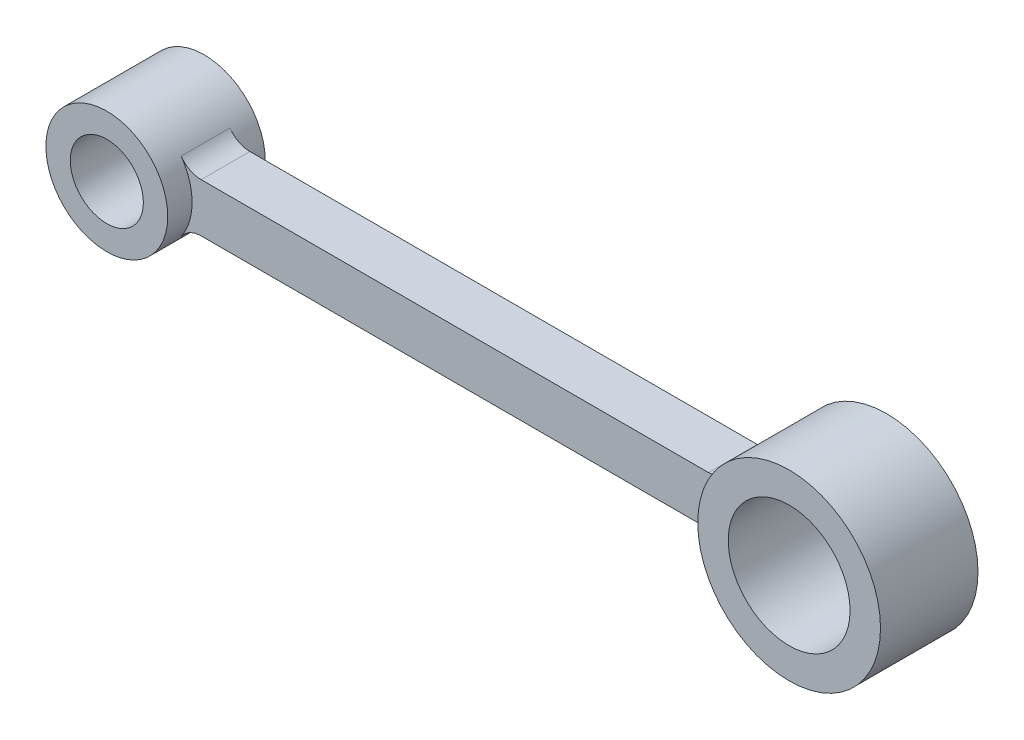
SolidWorks part; units mm, degrees
material "Plain Carbon Steel"
ref_plane "Front Plane" through (0, 0, 0) normal (0, 0, 1) x (1, 0, 0)
ref_plane "Top Plane" through (0, 0, 0) normal (0, 1, 0) x (1, 0, 0)
ref_plane "Right Plane" through (0, 0, 0) normal (1, 0, 0) x (0, 0, -1)
sketch "Rod Profile Sketch" plane through (0, 0, 0) normal (0, 0, 1) x (1, 0, 0)
  line L0 (-64.4606, 0) -> (30.4123, 0) construction
  line L1 (-34.25, 0) -> (-34.25, -9.9158) construction
  line L2 (34.25, 0) -> (34.25, -12.7494) construction
  circle A0 centre (-29.25, 0) radius 3
  circle A1 centre (-29.25, 0) radius 5
  circle A2 centre (26.75, 0) radius 5
  circle A3 centre (26.75, 0) radius 7.5
  dimension "D1" = 10
  dimension "D2" = 6
  dimension "D3" = 15
  dimension "D4" = 10
  dimension "D5" = 34.25
  dimension "D6" = 34.25
extrude "Rod Body Extrude 8mm" add sketch "Rod Profile Sketch" along normal mid plane 8
sketch "Shank Boss Sketch" plane through (0, 0, 0) normal (0, 0, 1) x (1, 0, 0)
  line L1 (-24.2751, -0.5) -> (36.528, -0.5) construction
  line L2 (-24.6674, 2) -> (19.5216, 2)
  line L4 (-24.6674, -2) -> (19.5216, -2)
  circle A0 centre (26.75, 0) radius 7.5 construction
  circle A1 centre (-29.25, 0) radius 5 construction
  arc A2 (19.5216, 2) -> (19.5216, -2) centre (26.75, 0) ccw
  arc A3 (-24.6674, -2) -> (-24.6674, 2) centre (-29.25, 0) ccw
  dimension "D1" = 2
  dimension "D2" = 4
  dimension "D3" = 1.5
extrude "Shank Boss 4mm" add sketch "Shank Boss Sketch" along normal mid plane 4
fillet "Shank Fillet R2" radius 2 4 edges at (19.5216, -2, 0) (19.5216, 2, 0) (-24.6674, -2, 0) (-24.6674, 2, 0)
